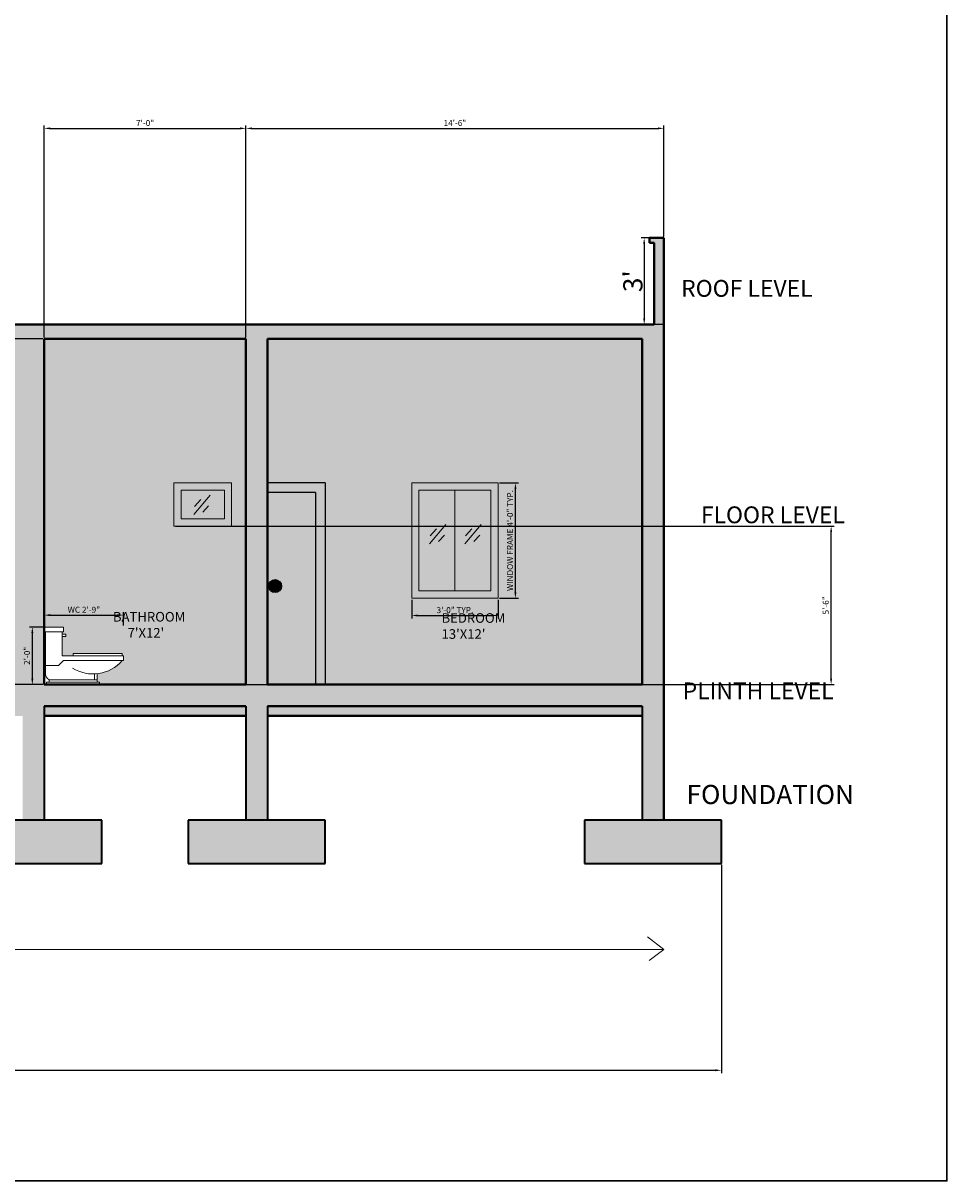
# Model space of a CAD drawing. Units: inches. Extents: x 2163 to 7246, y 928 to 2098.
# Tile 7 of 15: x 3249 to 3633, y 928 to 1411. Entities that reach past the tile are written whole.
import ezdxf

# ---------------------------------------------------------------- set-up
doc = ezdxf.new("R2010")
doc.units = ezdxf.units.IN
for name, color, linetype, lineweight in [('A-ANNO-DIMS', 4, 'Continuous', 18), ('A-ANNO-TEXT', 7, 'Continuous', 18), ('A-ANNO-TTLB', 7, 'Continuous', 30), ('A-AREA-IDEN', 7, 'Continuous', 18), ('A-DOOR', 4, 'Continuous', 25), ('A-DOOR-PATT', 35, 'Continuous', 9), ('A-FLOR-FIXT', 9, 'Continuous', 20), ('A-GLAZ', 30, 'Continuous', 20), ('A-SECT', 7, 'Continuous', 40), ('A-SECT-CUT-PATT', 250, 'Continuous', 13), ('S-FNDN', 7, 'Continuous', 35), ('S-FNDN-PATT', 252, 'Continuous', 13)]:
    doc.layers.add(name, color=color, linetype=linetype, lineweight=lineweight)
doc.layers.add('A-GLAZ-PATT', color=141, linetype='Continuous', lineweight=9, true_color=0xadddf7)
doc.layers.add('A-SECT-PATT', color=51, linetype='Continuous', lineweight=9, true_color=0xf8f6b0)
doc.styles.get("Standard").update_dxf_attribs({"font": 'arial.ttf'})
doc.dimstyles.new('ISO-25', dxfattribs={"dimtxt": 2.5, "dimasz": 2.5, "dimexe": 1.25, "dimexo": 0.625, "dimtad": 1, "dimdec": 0, "dimlunit": 3, "dimtxsty": 'Standard', "dimcen": 2.5, "dimadec": 0, "dimazin": 0, "dimtfac": 1, "dimtdec": 0, "dimtmove": 0, "dimatfit": 3, "dimfxl": 1, "dimarcsym": 0})

# ---------------------------------------------------------------- blocks, each defined once
blk = doc.blocks.new('Toilet - side')
for p, q in [((0.5, 5), (0.5, 22)), ((7.5, 22), (7.5, 12)), ((7.5, 21), (9, 21)), ((9, 20), (7.5, 20)), ((9, 21), (9, 20)), ((8, 10), (6, 8)), ((7.5, 12), (33, 12)), ((33, 10), (8, 10)), ((32.5, 13), (12, 13)), ((12, 13), (12, 12)), ((32.5, 12), (32.5, 13)), ((33, 12), (33, 10)), ((6, 8), (0.5, 8)), ((22, 2), (2, 2)), ((2, 2), (2, 1)), ((21, 4.5), (21, 2)), ((22, 2), (22, 4.54)), ((22, 1), (22, 2))]:
    blk.add_line(p, q)
for points in [[(0, 22), (0, 24), (8, 24), (8, 22)], [(1, 0), (1, 1), (23, 1), (23, 0)]]:
    blk.add_lwpolyline(points, close=True)
for centre, radius, start, end in [((20.3, 20.7), 16.23, 238.1872, 318.7702), ((3.75, 4.75), 3.26, 175.6013, 237.5288)]:
    blk.add_arc(centre, radius, start, end)
blk = doc.blocks.new('*D28')
at = {"layer": 'A-ANNO-DIMS', "color": 0, "lineweight": -2, "transparency": 16777216}
for p, q in [((3514.92, 1321.11), (3506.1, 1321.11)), ((3507.35, 1318.61), (3507.35, 1287.61)), ((3514.92, 1285.11), (3506.1, 1285.11))]:
    blk.add_line(p, q, dxfattribs=at)
at = {"layer": 'A-ANNO-DIMS', "color": 0, "transparency": 16777216}
for points in [[(3506.94, 1318.61), (3507.77, 1318.61), (3507.35, 1321.11)], [(3506.94, 1287.61), (3507.77, 1287.61), (3507.35, 1285.11)]]:
    blk.add_solid(points, dxfattribs=at)
at = {"layer": 'Defpoints', "color": 0, "transparency": 16777216}
for p in [(3515.54, 1321.11), (3507.35, 1285.11), (3515.54, 1285.11)]:
    blk.add_point(p, dxfattribs=at)
at = {"layer": 'A-ANNO-DIMS', "color": 0, "transparency": 16777216, "insert": (3502.64, 1303.11), "char_height": 2.5, "attachment_point": 5, "rotation": 90}
blk.add_mtext("{\\H3.2x;3'}", dxfattribs=at)
blk = doc.blocks.new('FOOTING-57X18-SECTION')
for p, q in [((24, 18), (0, 18)), ((0, 18), (0, 0)), ((57, 18), (24, 18)), ((57, 0), (57, 18)), ((0, 0), (24, 0)), ((24, 0), (57, 0))]:
    blk.add_line(p, q)
blk = doc.blocks.new('WIN-36X48-FRAME-SECTION')
for p, q in [((0, 48), (36, 48)), ((0, 48), (0, 0)), ((3, 45), (33, 45)), ((3, 45), (3, 3)), ((18, 45), (18, 3)), ((33, 45), (33, 3)), ((36, 48), (36, 0)), ((0, 0), (36, 0)), ((3, 3), (33, 3))]:
    blk.add_line(p, q)
blk = doc.blocks.new('DOOR-FRAME-SECTION')
for p, q in [((0, 84), (0, 0)), ((0, 84), (24, 84)), ((4, 80), (24, 80)), ((4, 80), (4, 0))]:
    blk.add_line(p, q)
blk = doc.blocks.new('GLAZ-REFLECTION-SECTION')
for p, q in [((0, 0), (6.77, 8.07)), ((0.29, 3.36), (2.9, 6.25)), ((3.76, 0.92), (6.2, 3.64))]:
    blk.add_line(p, q)
blk = doc.blocks.new('*D71')
at = {"layer": 'A-ANNO-DIMS', "color": 0, "lineweight": -2, "transparency": 16777216}
for p, q in [((3447.17, 1219.11), (3454.99, 1219.11)), ((3453.74, 1173.61), (3453.74, 1216.61)), ((3447.17, 1171.11), (3454.99, 1171.11))]:
    blk.add_line(p, q, dxfattribs=at)
at = {"layer": 'A-ANNO-DIMS', "color": 0, "transparency": 16777216}
for points in [[(3453.33, 1216.61), (3454.16, 1216.61), (3453.74, 1219.11)], [(3453.33, 1173.61), (3454.16, 1173.61), (3453.74, 1171.11)]]:
    blk.add_solid(points, dxfattribs=at)
at = {"layer": 'Defpoints', "color": 0, "transparency": 16777216}
for p in [(3446.54, 1219.11), (3453.74, 1219.11), (3446.54, 1171.11)]:
    blk.add_point(p, dxfattribs=at)
at = {"layer": 'A-ANNO-DIMS', "color": 0, "transparency": 16777216, "insert": (3451.83, 1195.11), "char_height": 2.5, "attachment_point": 5, "rotation": 90}
blk.add_mtext('WINDOW FRAME 4\'-0" TYP.', dxfattribs=at)
blk = doc.blocks.new('*D72')
at = {"layer": 'A-ANNO-DIMS', "color": 0, "lineweight": -2, "transparency": 16777216}
for p, q in [((3410.54, 1170.48), (3410.54, 1162.66)), ((3446.54, 1170.48), (3446.54, 1162.66)), ((3413.04, 1163.91), (3444.04, 1163.91))]:
    blk.add_line(p, q, dxfattribs=at)
at = {"layer": 'A-ANNO-DIMS', "color": 0, "transparency": 16777216}
for points in [[(3413.04, 1164.32), (3413.04, 1163.49), (3410.54, 1163.91)], [(3444.04, 1164.32), (3444.04, 1163.49), (3446.54, 1163.91)]]:
    blk.add_solid(points, dxfattribs=at)
at = {"layer": 'Defpoints', "color": 0, "transparency": 16777216}
for p in [(3410.54, 1171.11), (3446.54, 1171.11), (3446.54, 1163.91)]:
    blk.add_point(p, dxfattribs=at)
at = {"layer": 'A-ANNO-DIMS', "color": 0, "transparency": 16777216, "insert": (3428.54, 1165.81), "char_height": 2.5, "attachment_point": 5}
blk.add_mtext('3\'-0" TYP.', dxfattribs=at)
blk = doc.blocks.new('*D75')
at = {"layer": 'A-ANNO-DIMS', "color": 0, "lineweight": -2, "transparency": 16777216}
for p, q in [((3257.54, 1159.73), (3257.54, 1165.31)), ((3260.04, 1164.06), (3288.04, 1164.06)), ((3290.54, 1159.73), (3290.54, 1165.31))]:
    blk.add_line(p, q, dxfattribs=at)
at = {"layer": 'A-ANNO-DIMS', "color": 0, "transparency": 16777216}
for points in [[(3260.04, 1164.47), (3260.04, 1163.64), (3257.54, 1164.06)], [(3288.04, 1164.47), (3288.04, 1163.64), (3290.54, 1164.06)]]:
    blk.add_solid(points, dxfattribs=at)
at = {"layer": 'Defpoints', "color": 0, "transparency": 16777216}
for p in [(3290.54, 1164.06), (3257.54, 1159.11), (3290.54, 1159.11)]:
    blk.add_point(p, dxfattribs=at)
at = {"layer": 'A-ANNO-DIMS', "color": 0, "transparency": 16777216, "insert": (3274.04, 1165.97), "char_height": 2.5, "attachment_point": 5}
blk.add_mtext('WC 2\'-9"', dxfattribs=at)
blk = doc.blocks.new('*D76')
at = {"layer": 'A-ANNO-DIMS', "color": 0, "lineweight": -2, "transparency": 16777216}
for p, q in [((3256.92, 1159.11), (3251.34, 1159.11)), ((3252.59, 1137.61), (3252.59, 1156.61)), ((3256.92, 1135.11), (3251.34, 1135.11))]:
    blk.add_line(p, q, dxfattribs=at)
at = {"layer": 'A-ANNO-DIMS', "color": 0, "transparency": 16777216}
for points in [[(3252.18, 1156.61), (3253.01, 1156.61), (3252.59, 1159.11)], [(3252.18, 1137.61), (3253.01, 1137.61), (3252.59, 1135.11)]]:
    blk.add_solid(points, dxfattribs=at)
at = {"layer": 'Defpoints', "color": 0, "transparency": 16777216}
for p in [(3252.59, 1159.11), (3257.54, 1159.11), (3257.54, 1135.11)]:
    blk.add_point(p, dxfattribs=at)
at = {"layer": 'A-ANNO-DIMS', "color": 0, "transparency": 16777216, "insert": (3250.69, 1147.11), "char_height": 2.5, "attachment_point": 5, "rotation": 90}
blk.add_mtext('2\'-0"', dxfattribs=at)
blk = doc.blocks.new('*D100')
at = {"layer": 'A-ANNO-DIMS', "color": 0, "lineweight": -2, "transparency": 16777216}
for p, q in [((2750.54, 1060.06), (2750.54, 973.27)), ((3539.54, 1060.06), (3539.54, 973.27)), ((2753.04, 974.52), (3537.04, 974.52))]:
    blk.add_line(p, q, dxfattribs=at)
at = {"layer": 'A-ANNO-DIMS', "color": 0, "transparency": 16777216}
for points in [[(2753.04, 974.94), (2753.04, 974.11), (2750.54, 974.52)], [(3537.04, 974.94), (3537.04, 974.11), (3539.54, 974.52)]]:
    blk.add_solid(points, dxfattribs=at)
at = {"layer": 'Defpoints', "color": 0, "transparency": 16777216}
for p in [(2750.54, 1060.68), (3539.54, 1060.68), (3539.54, 974.52)]:
    blk.add_point(p, dxfattribs=at)
at = {"layer": 'A-ANNO-DIMS', "color": 0, "transparency": 16777216, "insert": (3145.04, 976.42), "char_height": 2.5, "attachment_point": 5}
blk.add_mtext('65\'-9"', dxfattribs=at)
blk = doc.blocks.new('*D105')
at = {"layer": 'A-ANNO-DIMS', "color": 0, "lineweight": -2, "transparency": 16777216}
for p, q in [((3341.54, 1279.73), (3341.54, 1368.01)), ((3344.04, 1366.76), (3513.04, 1366.76)), ((3515.54, 1321.73), (3515.54, 1368.01))]:
    blk.add_line(p, q, dxfattribs=at)
at = {"layer": 'A-ANNO-DIMS', "color": 0, "transparency": 16777216}
for points in [[(3344.04, 1367.17), (3344.04, 1366.34), (3341.54, 1366.76)], [(3513.04, 1367.17), (3513.04, 1366.34), (3515.54, 1366.76)]]:
    blk.add_solid(points, dxfattribs=at)
at = {"layer": 'Defpoints', "color": 0, "transparency": 16777216}
for p in [(3515.54, 1366.76), (3515.54, 1321.11), (3341.54, 1279.11)]:
    blk.add_point(p, dxfattribs=at)
at = {"layer": 'A-ANNO-DIMS', "color": 0, "transparency": 16777216, "insert": (3428.54, 1368.66), "char_height": 2.5, "attachment_point": 5}
blk.add_mtext('14\'-6"', dxfattribs=at)
blk = doc.blocks.new('*D106')
at = {"layer": 'A-ANNO-DIMS', "color": 0, "lineweight": -2, "transparency": 16777216}
for p, q in [((3257.54, 1279.73), (3257.54, 1368.01)), ((3260.04, 1366.76), (3339.04, 1366.76)), ((3341.54, 1279.73), (3341.54, 1368.01))]:
    blk.add_line(p, q, dxfattribs=at)
at = {"layer": 'A-ANNO-DIMS', "color": 0, "transparency": 16777216}
for points in [[(3260.04, 1367.17), (3260.04, 1366.34), (3257.54, 1366.76)], [(3339.04, 1367.17), (3339.04, 1366.34), (3341.54, 1366.76)]]:
    blk.add_solid(points, dxfattribs=at)
at = {"layer": 'Defpoints', "color": 0, "transparency": 16777216}
for p in [(3341.54, 1366.76), (3257.54, 1279.11), (3341.54, 1279.11)]:
    blk.add_point(p, dxfattribs=at)
at = {"layer": 'A-ANNO-DIMS', "color": 0, "transparency": 16777216, "insert": (3299.54, 1368.66), "char_height": 2.5, "attachment_point": 5}
blk.add_mtext('7\'-0"', dxfattribs=at)
blk = doc.blocks.new('*D107')
at = {"layer": 'A-ANNO-DIMS', "color": 0, "lineweight": -2, "transparency": 16777216}
for p, q in [((3256.92, 1279.11), (2663.63, 1279.11)), ((2664.88, 1137.61), (2664.88, 1276.61)), ((3256.92, 1135.11), (2663.63, 1135.11))]:
    blk.add_line(p, q, dxfattribs=at)
at = {"layer": 'A-ANNO-DIMS', "color": 0, "transparency": 16777216}
for points in [[(2664.46, 1276.61), (2665.3, 1276.61), (2664.88, 1279.11)], [(2664.46, 1137.61), (2665.3, 1137.61), (2664.88, 1135.11)]]:
    blk.add_solid(points, dxfattribs=at)
at = {"layer": 'Defpoints', "color": 0, "transparency": 16777216}
for p in [(2664.88, 1279.11), (3257.54, 1279.11), (3257.54, 1135.11)]:
    blk.add_point(p, dxfattribs=at)
at = {"layer": 'A-ANNO-DIMS', "color": 0, "transparency": 16777216, "insert": (2662.98, 1207.11), "char_height": 2.5, "attachment_point": 5, "rotation": 90}
blk.add_mtext('12\'-0"', dxfattribs=at)
blk = doc.blocks.new('*D108')
at = {"layer": 'A-ANNO-DIMS', "color": 0, "lineweight": -2, "transparency": 16777216}
for p, q in [((3312.17, 1201.11), (3586.44, 1201.11)), ((3585.19, 1137.61), (3585.19, 1198.61)), ((3258.17, 1135.11), (3586.44, 1135.11))]:
    blk.add_line(p, q, dxfattribs=at)
at = {"layer": 'A-ANNO-DIMS', "color": 0, "transparency": 16777216}
for points in [[(3584.78, 1198.61), (3585.61, 1198.61), (3585.19, 1201.11)], [(3584.78, 1137.61), (3585.61, 1137.61), (3585.19, 1135.11)]]:
    blk.add_solid(points, dxfattribs=at)
at = {"layer": 'Defpoints', "color": 0, "transparency": 16777216}
for p in [(3311.54, 1201.11), (3585.19, 1201.11), (3257.54, 1135.11)]:
    blk.add_point(p, dxfattribs=at)
at = {"layer": 'A-ANNO-DIMS', "color": 0, "transparency": 16777216, "insert": (3583.29, 1168.11), "char_height": 2.5, "attachment_point": 5, "rotation": 90}
blk.add_mtext('5\'-6"', dxfattribs=at)

msp = doc.modelspace()

# ---------------------------------------------------------------- hatches: boundary and pattern name
at = {"layer": 'A-DOOR-PATT'}
h = msp.add_hatch(color=256, dxfattribs=at)
h.dxf.hatch_style = 1
h.paths.add_polyline_path([(3350.54, 1219.11), (3350.54, 1215.11), (3370.54, 1215.11), (3370.54, 1135.11), (3374.54, 1135.11), (3374.54, 1219.11)])
h.paths.add_polyline_path([(3119.54, 1215.11), (3119.54, 1219.11), (3095.54, 1219.11), (3095.54, 1135.11), (3099.54, 1135.11), (3099.54, 1215.11)])
h.paths.add_polyline_path([(2923.54, 1215.11), (2923.54, 1219.11), (2899.54, 1219.11), (2899.54, 1135.11), (2903.54, 1135.11), (2903.54, 1215.11)])
h = msp.add_hatch(color=256, dxfattribs=at)
h.dxf.hatch_style = 1
h.paths.add_polyline_path([(2923.54, 1215.11), (2903.54, 1215.11), (2903.54, 1135.11), (2923.54, 1135.11)])
h.paths.add_polyline_path([(2921.06, 1176.14, -1), (2915.61, 1176.14, -1)], flags=16)
h.paths.add_polyline_path([(2920.22, 1176.14, -1), (2916.45, 1176.14, -1)], flags=0)
h.paths.add_polyline_path([(3099.54, 1135.11), (3119.54, 1135.11), (3119.54, 1215.11), (3099.54, 1215.11)])
h.paths.add_polyline_path([(3118.83, 1176.14, -1), (3113.38, 1176.14, -1)], flags=16)
h.paths.add_polyline_path([(3117.99, 1176.14, -1), (3114.22, 1176.14, -1)], flags=0)
h.paths.add_polyline_path([(3370.54, 1215.11), (3350.54, 1215.11), (3350.54, 1135.11), (3370.54, 1135.11)])
h.paths.add_polyline_path([(3356.37, 1176.14, -1), (3350.92, 1176.14, -1)], flags=16)
h.paths.add_polyline_path([(3355.53, 1176.14, -1), (3351.76, 1176.14, -1)], flags=0)
h = msp.add_hatch(color=256, dxfattribs=at)
h.dxf.hatch_style = 1
h.paths.add_polyline_path([(3350.92, 1176.14, 1), (3356.37, 1176.14, 1)])
h.paths.add_polyline_path([(3355.53, 1176.14, 1), (3351.76, 1176.14, 1)], flags=16)
h = msp.add_hatch(color=256, dxfattribs=at)
h.dxf.hatch_style = 1
h.paths.add_polyline_path([(3351.76, 1176.14, 1), (3355.53, 1176.14, 1)])
at = {"layer": 'A-GLAZ-PATT'}
h = msp.add_hatch(color=256, dxfattribs=at)
h.dxf.hatch_style = 1
h.paths.add_polyline_path([(2874.54, 1216.11), (2853.54, 1216.11), (2853.54, 1174.11), (2874.54, 1174.11)])
h.paths.add_polyline_path([(2853.54, 1216.11), (2832.54, 1216.11), (2832.54, 1174.11), (2853.54, 1174.11)])
h.paths.add_polyline_path([(3026.04, 1216.11), (2993.04, 1216.11), (2993.04, 1174.11), (3026.04, 1174.11)])
h.paths.add_polyline_path([(3059.04, 1216.11), (3026.04, 1216.11), (3026.04, 1174.11), (3059.04, 1174.11)])
h.paths.add_polyline_path([(3188.54, 1216.11), (3173.54, 1216.11), (3173.54, 1174.11), (3188.54, 1174.11)])
h.paths.add_polyline_path([(3203.54, 1216.11), (3188.54, 1216.11), (3188.54, 1174.11), (3203.54, 1174.11)])
h.paths.add_polyline_path([(3332.54, 1216.11), (3314.54, 1216.11), (3314.54, 1204.11), (3332.54, 1204.11)])
h.paths.add_polyline_path([(3428.54, 1216.11), (3413.54, 1216.11), (3413.54, 1174.11), (3428.54, 1174.11)])
h.paths.add_polyline_path([(3443.54, 1216.11), (3428.54, 1216.11), (3428.54, 1174.11), (3443.54, 1174.11)])
at = {"layer": 'A-SECT-CUT-PATT'}
h = msp.add_hatch(color=256, dxfattribs=at)
h.dxf.hatch_style = 1
h.paths.add_polyline_path([(2783.54, 1279.11), (2923.54, 1279.11), (2923.54, 1135.11), (2783.54, 1135.11), (2783.54, 1171.11), (2774.54, 1171.11), (2774.54, 1078.68), (2783.54, 1078.68), (2783.54, 1126.11), (2923.54, 1126.11), (2923.54, 1078.68), (2932.54, 1078.68), (2932.54, 1126.11), (3119.54, 1126.11), (3119.54, 1078.68), (3128.54, 1078.68), (3128.54, 1126.11), (3248.54, 1126.11), (3248.54, 1078.68), (3257.54, 1078.68), (3257.54, 1126.11), (3341.54, 1126.11), (3341.54, 1078.68), (3350.54, 1078.68), (3350.54, 1126.11), (3506.54, 1126.11), (3506.54, 1078.68), (3515.54, 1078.68), (3515.54, 1321.11), (3511.54, 1321.11), (3509.54, 1321.11), (3509.54, 1319.11), (3511.54, 1319.11), (3511.54, 1285.11), (2778.54, 1285.11), (2778.54, 1319.11), (2780.54, 1319.11), (2780.54, 1321.11), (2778.54, 1321.11), (2774.54, 1321.11), (2774.54, 1219.11), (2783.54, 1219.11)])
h.paths.add_polyline_path([(2932.54, 1279.11), (3119.54, 1279.11), (3119.54, 1135.11), (2932.54, 1135.11)], flags=16)
h.paths.add_polyline_path([(2990.04, 1219.11), (3062.04, 1219.11), (3062.04, 1171.11), (2990.04, 1171.11)], flags=0)
h.paths.add_polyline_path([(2993.04, 1216.11), (3059.04, 1216.11), (3059.04, 1174.11), (2993.04, 1174.11)], flags=0)
h.paths.add_polyline_path([(3118.83, 1176.14, -1), (3113.38, 1176.14, -1)], flags=0)
h.paths.add_polyline_path([(3117.99, 1176.14, -1), (3114.22, 1176.14, -1)], flags=0)
h.paths.add_polyline_path([(3128.54, 1279.11), (3248.54, 1279.11), (3248.54, 1135.11), (3128.54, 1135.11)], flags=16)
h.paths.add_polyline_path([(3170.54, 1219.11), (3206.54, 1219.11), (3206.54, 1171.11), (3170.54, 1171.11)], flags=0)
h.paths.add_polyline_path([(3173.54, 1216.11), (3203.54, 1216.11), (3203.54, 1174.11), (3173.54, 1174.11)], flags=0)
h.paths.add_polyline_path([(3257.54, 1279.11), (3341.54, 1279.11), (3341.54, 1135.11), (3257.54, 1135.11)], flags=16)
h.paths.add_polyline_path([(3257.54, 1159.11), (3265.54, 1159.11), (3265.54, 1157.11), (3265.04, 1157.11), (3265.04, 1156.11), (3266.54, 1156.11), (3266.54, 1155.11), (3265.04, 1155.11), (3265.04, 1147.11), (3269.54, 1147.11), (3269.54, 1148.11), (3290.04, 1148.11), (3290.04, 1147.11), (3290.54, 1147.11), (3290.54, 1145.11), (3290.04, 1145.11, -0.188679), (3279.54, 1139.66), (3279.54, 1137.11), (3279.54, 1136.11), (3280.54, 1136.11), (3280.54, 1135.11), (3258.54, 1135.11), (3258.54, 1136.11), (3259.54, 1136.11), (3259.54, 1137.11), (3278.54, 1137.11), (3278.54, 1139.59, 0.204728), (3290.04, 1145.11), (3265.54, 1145.11), (3263.54, 1143.11), (3258.04, 1143.11), (3258.04, 1157.11), (3257.54, 1157.11)], flags=0)
h.paths.add_polyline_path([(3311.54, 1219.11), (3335.54, 1219.11), (3335.54, 1201.11), (3311.54, 1201.11)], flags=0)
h.paths.add_polyline_path([(3314.54, 1216.11), (3332.54, 1216.11), (3332.54, 1204.11), (3314.54, 1204.11)], flags=0)
h.paths.add_polyline_path([(3350.54, 1279.11), (3506.54, 1279.11), (3506.54, 1135.11), (3350.54, 1135.11)], flags=16)
h.paths.add_polyline_path([(3356.37, 1176.14, -1), (3350.92, 1176.14, -1)], flags=0)
h.paths.add_polyline_path([(3355.53, 1176.14, -1), (3351.76, 1176.14, -1)], flags=0)
h.paths.add_polyline_path([(3410.54, 1219.11), (3446.54, 1219.11), (3446.54, 1171.11), (3410.54, 1171.11)], flags=0)
h.paths.add_polyline_path([(3413.54, 1216.11), (3443.54, 1216.11), (3443.54, 1174.11), (3413.54, 1174.11)], flags=0)
h = msp.add_hatch(color=256, dxfattribs=at)
h.dxf.hatch_style = 1
h.paths.add_polyline_path([(2783.54, 1216.11), (2783.54, 1219.11), (2774.54, 1219.11), (2774.54, 1216.11)])
h.paths.add_polyline_path([(2774.54, 1174.11), (2774.54, 1171.11), (2783.54, 1171.11), (2783.54, 1174.11)])
h.paths.add_polyline_path([(2877.54, 1171.11), (2877.54, 1219.11), (2829.54, 1219.11), (2829.54, 1171.11)])
h.paths.add_polyline_path([(2832.54, 1174.11), (2832.54, 1216.11), (2874.54, 1216.11), (2874.54, 1174.11)], flags=16)
h.paths.add_polyline_path([(3062.04, 1171.11), (3062.04, 1219.11), (2990.04, 1219.11), (2990.04, 1171.11)])
h.paths.add_polyline_path([(2993.04, 1174.11), (2993.04, 1216.11), (3059.04, 1216.11), (3059.04, 1174.11)], flags=16)
h.paths.add_polyline_path([(3206.54, 1171.11), (3206.54, 1219.11), (3170.54, 1219.11), (3170.54, 1171.11)])
h.paths.add_polyline_path([(3173.54, 1174.11), (3173.54, 1216.11), (3203.54, 1216.11), (3203.54, 1174.11)], flags=16)
h.paths.add_polyline_path([(3335.54, 1201.11), (3335.54, 1219.11), (3311.54, 1219.11), (3311.54, 1201.11)])
h.paths.add_polyline_path([(3314.54, 1204.11), (3314.54, 1216.11), (3332.54, 1216.11), (3332.54, 1204.11)], flags=16)
h.paths.add_polyline_path([(3446.54, 1171.11), (3446.54, 1219.11), (3410.54, 1219.11), (3410.54, 1171.11)])
h.paths.add_polyline_path([(3413.54, 1174.11), (3413.54, 1216.11), (3443.54, 1216.11), (3443.54, 1174.11)], flags=16)
at = {"layer": 'A-SECT-PATT'}
h = msp.add_hatch(color=256, dxfattribs=at)
h.dxf.hatch_style = 1
h.paths.add_polyline_path([(2783.54, 1279.11), (2783.54, 1135.11), (2899.54, 1135.11), (2899.54, 1219.11), (2923.54, 1219.11), (2923.54, 1279.11)])
h.paths.add_polyline_path([(2877.54, 1219.11), (2877.54, 1171.11), (2829.54, 1171.11), (2829.54, 1219.11)], flags=16)
h.paths.add_polyline_path([(2874.54, 1216.11), (2874.54, 1174.11), (2832.54, 1174.11), (2832.54, 1216.11)], flags=0)
h.paths.add_polyline_path([(2932.54, 1279.11), (2932.54, 1135.11), (3095.54, 1135.11), (3095.54, 1219.11), (3119.54, 1219.11), (3119.54, 1279.11)])
h.paths.add_polyline_path([(3062.04, 1219.11), (3062.04, 1171.11), (2990.04, 1171.11), (2990.04, 1219.11)], flags=16)
h.paths.add_polyline_path([(3059.04, 1216.11), (3059.04, 1174.11), (2993.04, 1174.11), (2993.04, 1216.11)], flags=0)
h.paths.add_polyline_path([(3128.54, 1135.11), (3248.54, 1135.11), (3248.54, 1279.11), (3128.54, 1279.11)])
h.paths.add_polyline_path([(3170.54, 1219.11), (3206.54, 1219.11), (3206.54, 1171.11), (3170.54, 1171.11)], flags=16)
h.paths.add_polyline_path([(3173.54, 1216.11), (3203.54, 1216.11), (3203.54, 1174.11), (3173.54, 1174.11)], flags=0)
h.paths.add_polyline_path([(3257.54, 1159.11), (3265.54, 1159.11), (3265.54, 1157.11), (3265.04, 1157.11), (3265.04, 1156.11), (3266.54, 1156.11), (3266.54, 1155.11), (3265.04, 1155.11), (3265.04, 1147.11), (3269.54, 1147.11), (3269.54, 1148.11), (3290.04, 1148.11), (3290.04, 1147.11), (3290.54, 1147.11), (3290.54, 1145.11), (3290.04, 1145.11, -0.188679), (3279.54, 1139.66), (3279.54, 1137.11), (3279.54, 1136.11), (3280.54, 1136.11), (3280.54, 1135.11), (3341.54, 1135.11), (3341.54, 1279.11), (3257.54, 1279.11)])
h.paths.add_polyline_path([(3311.54, 1219.11), (3335.54, 1219.11), (3335.54, 1201.11), (3311.54, 1201.11)], flags=16)
h.paths.add_polyline_path([(3314.54, 1216.11), (3332.54, 1216.11), (3332.54, 1204.11), (3314.54, 1204.11)], flags=0)
h.paths.add_polyline_path([(3350.54, 1279.11), (3350.54, 1219.11), (3374.54, 1219.11), (3374.54, 1135.11), (3506.54, 1135.11), (3506.54, 1279.11)])
h.paths.add_polyline_path([(3446.54, 1219.11), (3446.54, 1171.11), (3410.54, 1171.11), (3410.54, 1219.11)], flags=16)
h.paths.add_polyline_path([(3443.54, 1216.11), (3443.54, 1174.11), (3413.54, 1174.11), (3413.54, 1216.11)], flags=0)
h.paths.add_polyline_path([(2835.76, 1152.2), (2883.7, 1152.2), (2883.7, 1167.12), (2835.76, 1167.12)], flags=24)
h.paths.add_polyline_path([(3019.5, 1152.59), (3045.3, 1152.59), (3045.3, 1167.51), (3019.5, 1167.51)], flags=24)
h.paths.add_polyline_path([(3180.22, 1151.37), (3206.95, 1151.37), (3206.95, 1166.3), (3180.22, 1166.3)], flags=24)
h.paths.add_polyline_path([(3284.73, 1152.43), (3319.02, 1152.43), (3319.02, 1167.36), (3284.73, 1167.36)], flags=24)
h.paths.add_polyline_path([(3421.37, 1151.92), (3452.45, 1151.92), (3452.45, 1166.85), (3421.37, 1166.85)], flags=24)
at = {"layer": 'S-FNDN-PATT'}
h = msp.add_hatch(color=256, dxfattribs=at)
h.dxf.hatch_style = 1
h.paths.add_polyline_path([(2783.54, 1126.11), (2783.54, 1122.11), (2923.54, 1122.11), (2923.54, 1126.11)])
h.paths.add_polyline_path([(2932.54, 1126.11), (2932.54, 1122.11), (3119.54, 1122.11), (3119.54, 1126.11)])
h.paths.add_polyline_path([(3128.54, 1126.11), (3128.54, 1122.11), (3248.54, 1122.11), (3248.54, 1126.11)])
h.paths.add_polyline_path([(3341.54, 1122.11), (3341.54, 1126.11), (3257.54, 1126.11), (3257.54, 1122.11)])
h.paths.add_polyline_path([(3350.54, 1126.11), (3350.54, 1122.11), (3506.54, 1122.11), (3506.54, 1126.11)])
h = msp.add_hatch(color=256, dxfattribs=at)
h.dxf.hatch_style = 1
h.paths.add_polyline_path([(2807.54, 1060.68), (2807.54, 1078.68), (2774.54, 1078.68), (2750.54, 1078.68), (2750.54, 1060.68), (2774.54, 1060.68)])
h.paths.add_polyline_path([(2923.54, 1060.68), (2956.54, 1060.68), (2956.54, 1078.68), (2923.54, 1078.68), (2899.54, 1078.68), (2899.54, 1060.68)])
h.paths.add_polyline_path([(3119.54, 1060.68), (3152.54, 1060.68), (3152.54, 1078.68), (3119.54, 1078.68), (3095.54, 1078.68), (3095.54, 1060.68)])
h.paths.add_polyline_path([(3248.54, 1078.68), (3224.54, 1078.68), (3224.54, 1060.68), (3248.54, 1060.68), (3281.54, 1060.68), (3281.54, 1078.68)])
h.paths.add_polyline_path([(3374.54, 1060.68), (3374.54, 1078.68), (3341.54, 1078.68), (3317.54, 1078.68), (3317.54, 1060.68), (3341.54, 1060.68)])
h.paths.add_polyline_path([(3539.54, 1060.68), (3539.54, 1078.68), (3506.54, 1078.68), (3482.54, 1078.68), (3482.54, 1060.68), (3506.54, 1060.68)])

# ---------------------------------------------------------------- linework, layer by layer
at = {"layer": 'A-ANNO-DIMS'}
for p, q in [((3515.54, 1024.87), (3508.75, 1030.1)), ((2774.54, 1024.87), (3515.54, 1024.87)), ((3515.54, 1024.87), (3509.4, 1020.17))]:
    msp.add_line(p, q, dxfattribs=at)
at = {"layer": 'A-ANNO-TTLB'}
msp.add_lwpolyline([(2162.62, 2098.21), (3633.38, 2098.21), (3633.38, 928.48), (2162.62, 928.48)], close=True, dxfattribs=at)
at = {"layer": 'A-DOOR'}
for radius in [2.72, 1.89]:
    msp.add_circle((3353.65, 1176.14), radius, dxfattribs=at)
at = {"layer": 'A-GLAZ'}
for p, q in [((3335.54, 1219.11), (3311.54, 1219.11)), ((3311.54, 1219.11), (3311.54, 1201.11)), ((3314.54, 1216.11), (3314.54, 1204.11)), ((3332.54, 1216.11), (3314.54, 1216.11)), ((3332.54, 1216.11), (3332.54, 1204.11)), ((3335.54, 1219.11), (3335.54, 1201.11)), ((3311.54, 1201.11), (3335.54, 1201.11)), ((3314.54, 1204.11), (3332.54, 1204.11))]:
    msp.add_line(p, q, dxfattribs=at)
at = {"layer": 'A-SECT'}
for p, q in [((3511.54, 1321.11), (3509.54, 1321.11)), ((3509.54, 1321.11), (3509.54, 1319.11)), ((3511.54, 1321.11), (3515.54, 1321.11)), ((3515.54, 1321.11), (3515.54, 1078.68)), ((3509.54, 1319.11), (3511.54, 1319.11)), ((3511.54, 1319.11), (3511.54, 1285.11)), ((2778.54, 1285.11), (3511.54, 1285.11)), ((3257.54, 1279.11), (3257.54, 1135.11)), ((3257.54, 1279.11), (3341.54, 1279.11)), ((3341.54, 1279.11), (3341.54, 1135.11)), ((3350.54, 1279.11), (3350.54, 1135.11)), ((3350.54, 1279.11), (3506.54, 1279.11)), ((3506.54, 1279.11), (3506.54, 1135.11)), ((3257.54, 1135.11), (3341.54, 1135.11)), ((3350.54, 1135.11), (3506.54, 1135.11)), ((3257.54, 1126.11), (3341.54, 1126.11)), ((3350.54, 1126.11), (3506.54, 1126.11)), ((3257.54, 1122.11), (3341.54, 1122.11)), ((3350.54, 1122.11), (3506.54, 1122.11))]:
    msp.add_line(p, q, dxfattribs=at)
at = {"layer": 'S-FNDN'}
for p, q in [((3257.54, 1126.11), (3257.54, 1078.68)), ((3341.54, 1126.11), (3341.54, 1078.68)), ((3350.54, 1126.11), (3350.54, 1078.68)), ((3506.54, 1126.11), (3506.54, 1078.68))]:
    msp.add_line(p, q, dxfattribs=at)

# ---------------------------------------------------------------- block references
at = {"layer": 'A-DOOR', "extrusion": (0, 0, -1), "zscale": -1}
msp.add_blockref('DOOR-FRAME-SECTION', (-3374.54, 1135.11), dxfattribs=at)
at = {"layer": 'A-FLOR-FIXT'}
msp.add_blockref('Toilet - side', (3257.54, 1135.11), dxfattribs=at)
at = {"layer": 'A-GLAZ'}
for name, p in [('WIN-36X48-FRAME-SECTION', (3410.54, 1171.11)), ('GLAZ-REFLECTION-SECTION', (3319.8, 1205.95)), ('GLAZ-REFLECTION-SECTION', (3418, 1193.76)), ('GLAZ-REFLECTION-SECTION', (3432.66, 1193.76))]:
    msp.add_blockref(name, p, dxfattribs=at)
at = {"layer": 'S-FNDN'}
for p in [(3224.54, 1060.68), (3317.54, 1060.68), (3482.54, 1060.68)]:
    msp.add_blockref('FOOTING-57X18-SECTION', p, dxfattribs=at)

# ---------------------------------------------------------------- texts
at = {"layer": 'A-ANNO-TEXT', "attachment_point": 1}
for s, width, insert, char_height in [('ROOF LEVEL', 134.4138, (3522.73, 1303.63), 7), ('FLOOR LEVEL', 197.3337, (3530.96, 1209.33), 7), ('PLINTH LEVEL', 149.2532, (3523.38, 1136.01), 7), ('FOUNDATION', 343.0602, (3524.98, 1093.37), 8)]:
    msp.add_mtext_dynamic_manual_height_columns(s, width=width, gutter_width=12.5, heights=[0], dxfattribs=dict(at, insert=insert, char_height=char_height))
at = {"layer": 'A-AREA-IDEN', "char_height": 4, "attachment_point": 1}
for s, insert in [("BATHROOM\\P     7'X12'", (3286.14, 1165.37)), ("BEDROOM\\P13'X12'", (3422.98, 1164.86))]:
    msp.add_mtext_dynamic_manual_height_columns(s, width=30.4837, gutter_width=12.5, heights=[0], dxfattribs=dict(at, insert=insert))

# ---------------------------------------------------------------- dimensions: what is measured, and where the dimension line sits
at = {"layer": 'A-ANNO-DIMS'}
for base, p1, p2, picture, middle in [((3341.54, 1366.76), (3257.54, 1279.11), (3341.54, 1279.11), '*D106', (3299.54, 1368.66)), ((3515.54, 1366.76), (3341.54, 1279.11), (3515.54, 1321.11), '*D105', (3428.54, 1368.66)), ((3539.54, 974.52), (2750.54, 1060.68), (3539.54, 1060.68), '*D100', (3145.04, 976.42))]:
    dim = msp.add_linear_dim(base=base, p1=p1, p2=p2, dimstyle='ISO-25', override={"dimdec": 1, "dimlfac": 1, "dimrnd": 0, "dimzin": 1, "dimdsep": 46, "dimlunit": 4, "dimfrac": 2}, dxfattribs=at)
    dim.commit()
    dim.dimension.update_dxf_attribs({"geometry": picture, "text_midpoint": middle})
for base, p1, p2, text, override, picture, middle in [((3507.35, 1285.11), (3515.54, 1321.11), (3515.54, 1285.11), '{\\H3.2x;<>}', {"dimclrd": 0, "dimclre": 0, "dimclrt": 0}, '*D28', (3502.64, 1303.11)), ((3453.74, 1219.11), (3446.54, 1171.11), (3446.54, 1219.11), 'WINDOW FRAME <> TYP.', {"dimdec": 1, "dimlfac": 1, "dimrnd": 0, "dimzin": 1, "dimdsep": 46, "dimlunit": 4, "dimfrac": 2}, '*D71', (3451.83, 1195.11))]:
    dim = msp.add_linear_dim(base=base, p1=p1, p2=p2, angle=90, text=text, dimstyle='ISO-25', override=override, dxfattribs=at)
    dim.commit()
    dim.dimension.update_dxf_attribs({"geometry": picture, "text_midpoint": middle})
for base, p2, picture, middle in [((2664.88, 1279.11), (3257.54, 1279.11), '*D107', (2662.98, 1207.11)), ((3585.19, 1201.11), (3311.54, 1201.11), '*D108', (3583.29, 1168.11)), ((3252.59, 1159.11), (3257.54, 1159.11), '*D76', (3250.69, 1147.11))]:
    dim = msp.add_linear_dim(base=base, p1=(3257.54, 1135.11), p2=p2, angle=90, dimstyle='ISO-25', override={"dimdec": 1, "dimlfac": 1, "dimrnd": 0, "dimzin": 1, "dimdsep": 46, "dimlunit": 4, "dimfrac": 2}, dxfattribs=at)
    dim.commit()
    dim.dimension.update_dxf_attribs({"geometry": picture, "text_midpoint": middle})
for base, p1, p2, text, picture, middle in [((3290.54, 1164.06), (3257.54, 1159.11), (3290.54, 1159.11), 'WC <>', '*D75', (3274.04, 1165.97)), ((3446.54, 1163.91), (3410.54, 1171.11), (3446.54, 1171.11), '<> TYP.', '*D72', (3428.54, 1165.81))]:
    dim = msp.add_linear_dim(base=base, p1=p1, p2=p2, text=text, dimstyle='ISO-25', override={"dimdec": 1, "dimlfac": 1, "dimrnd": 0, "dimzin": 1, "dimdsep": 46, "dimlunit": 4, "dimfrac": 2}, dxfattribs=at)
    dim.commit()
    dim.dimension.update_dxf_attribs({"geometry": picture, "text_midpoint": middle})

doc.saveas('drawing.dxf')
